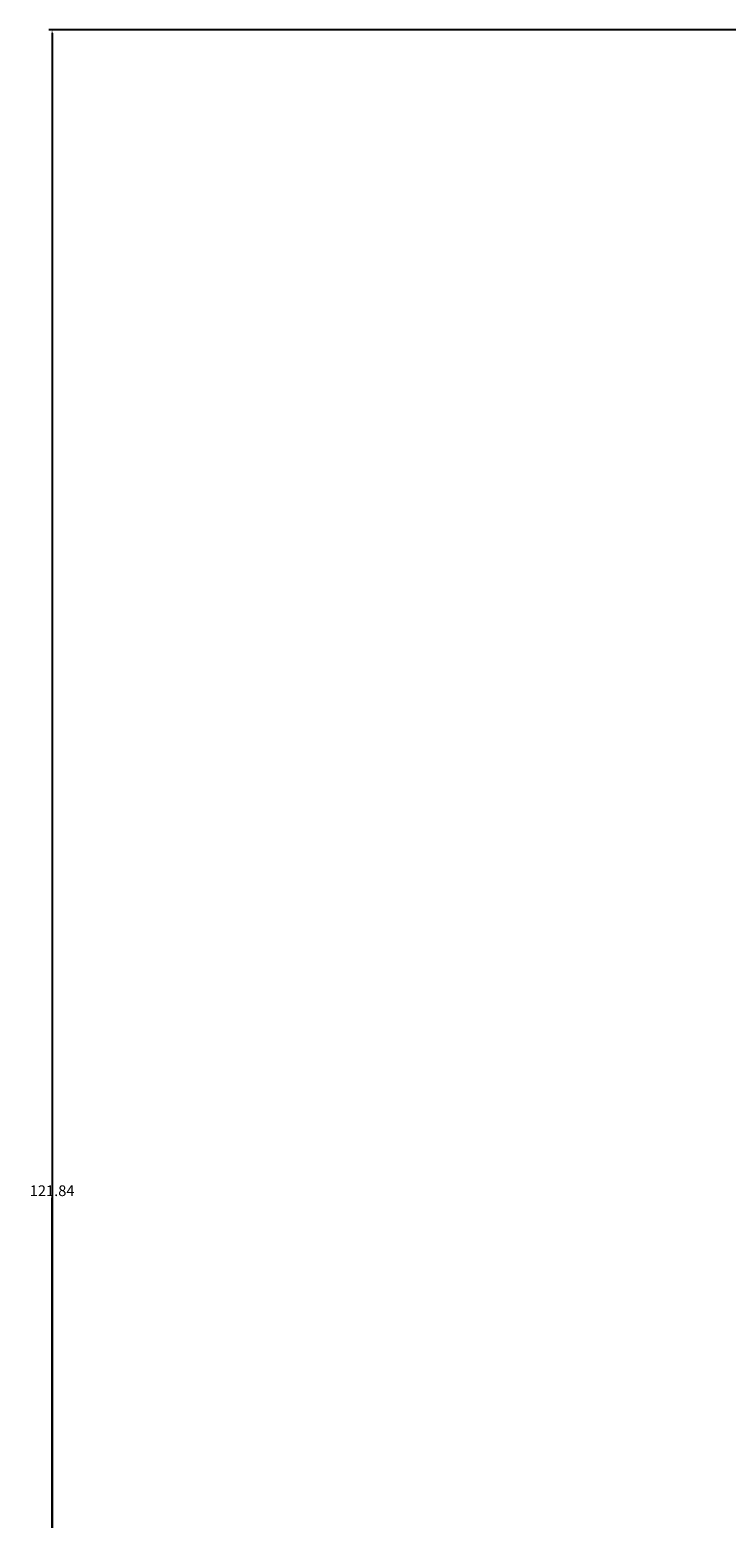
# Model space of a CAD drawing. Units: inches. Extents: x -26 to 776, y -22 to 650.
# Tile 29 of 62: x -26 to 10, y 535 to 613. Entities that reach past the tile are written whole.
import ezdxf

# ---------------------------------------------------------------- set-up
doc = ezdxf.new("R2010")
doc.units = ezdxf.units.IN
doc.header["$MEASUREMENT"] = 0
doc.layers.add('A-ANNO-DIMS', color=2, linetype='Continuous', lineweight=18)
doc.styles.get("Standard").update_dxf_attribs({"font": 'arial.ttf'})
doc.dimstyles.get("Standard").update_dxf_attribs({"dimtxt": 0.5625, "dimasz": 0.18, "dimexe": 0.18, "dimexo": 0.0625, "dimgap": 0.09, "dimtad": 0, "dimtih": 1, "dimtoh": 1, "dimdec": 4, "dimzin": 0, "dimdsep": 46, "dimlunit": 4, "dimtxsty": 'Standard', "dimcen": 0.09, "dimadec": 0, "dimazin": 0, "dimtfac": 1, "dimtdec": 4, "dimtofl": 0, "dimtmove": 0, "dimatfit": 3, "dimfxl": 1, "dimtolj": 1, "dimtzin": 0, "dimarcsym": 0})

# ---------------------------------------------------------------- blocks, each defined once
blk = doc.blocks.new('*D14')
at = {"layer": 'A-ANNO-DIMS', "color": 0, "lineweight": -2, "transparency": 16777216}
for p, q in [((191.616, 613.271), (-25.478, 613.271)), ((-25.298, 613.091), (-25.298, 314.754)), ((-25.298, 15.662), (-25.298, 314)), ((11.045, 15.482), (-25.478, 15.482))]:
    blk.add_line(p, q, dxfattribs=at)
at = {"layer": 'A-ANNO-DIMS', "color": 0, "transparency": 16777216}
for points in [[(-25.328, 613.091), (-25.268, 613.091), (-25.298, 613.271)], [(-25.328, 15.662), (-25.268, 15.662), (-25.298, 15.482)]]:
    blk.add_solid(points, dxfattribs=at)
at = {"layer": 'Defpoints', "color": 0, "transparency": 16777216}
for p in [(-25.298, 613.271), (191.678, 613.271), (11.107, 15.482)]:
    blk.add_point(p, dxfattribs=at)
at = {"layer": 'A-ANNO-DIMS', "color": 0, "transparency": 16777216, "insert": (-25.298, 314.377), "char_height": 0.5625, "attachment_point": 5}
blk.add_mtext('\\A1;597.8', dxfattribs=at)
blk = doc.blocks.new('*D19')
at = {"layer": 'A-ANNO-DIMS', "color": 0, "lineweight": -2, "transparency": 16777216}
for p, q in [((191.616, 613.271), (-25.478, 613.271)), ((-25.298, 613.091), (-25.298, 552.726)), ((-25.298, 491.607), (-25.298, 551.972)), ((191.616, 491.427), (-25.478, 491.427))]:
    blk.add_line(p, q, dxfattribs=at)
at = {"layer": 'A-ANNO-DIMS', "color": 0, "transparency": 16777216}
for points in [[(-25.328, 613.091), (-25.268, 613.091), (-25.298, 613.271)], [(-25.328, 491.607), (-25.268, 491.607), (-25.298, 491.427)]]:
    blk.add_solid(points, dxfattribs=at)
at = {"layer": 'Defpoints', "color": 0, "transparency": 16777216}
for p in [(-25.298, 613.271), (191.678, 613.271), (191.678, 491.427)]:
    blk.add_point(p, dxfattribs=at)
at = {"layer": 'A-ANNO-DIMS', "color": 0, "transparency": 16777216, "insert": (-25.298, 552.349), "char_height": 0.5625, "attachment_point": 5}
blk.add_mtext('\\A1;121.84', dxfattribs=at)

msp = doc.modelspace()

# ---------------------------------------------------------------- dimensions: what is measured, and where the dimension line sits
at = {"layer": 'A-ANNO-DIMS'}
for p1, override, picture, middle in [((191.6782, 491.4269), {"dimdec": 2, "dimlfac": 1, "dimrnd": 0, "dimzin": 0, "dimdsep": 46, "dimlunit": 2}, '*D19', (-25.2976, 552.3491)), ((11.1074, 15.4824), {"dimdec": 1, "dimlfac": 1, "dimrnd": 0, "dimzin": 0, "dimdsep": 46, "dimlunit": 2}, '*D14', (-25.2976, 314.3769))]:
    dim = msp.add_linear_dim(base=(-25.2976, 613.2713), p1=p1, p2=(191.6782, 613.2713), angle=90, dimstyle='Standard', override=override, dxfattribs=at)
    dim.commit()
    dim.dimension.update_dxf_attribs({"geometry": picture, "text_midpoint": middle})

doc.saveas('drawing.dxf')
